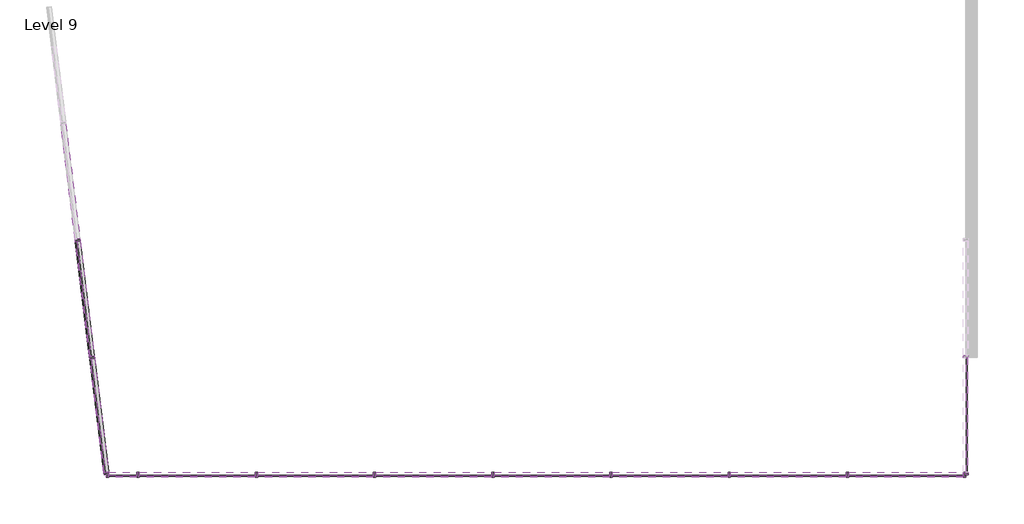
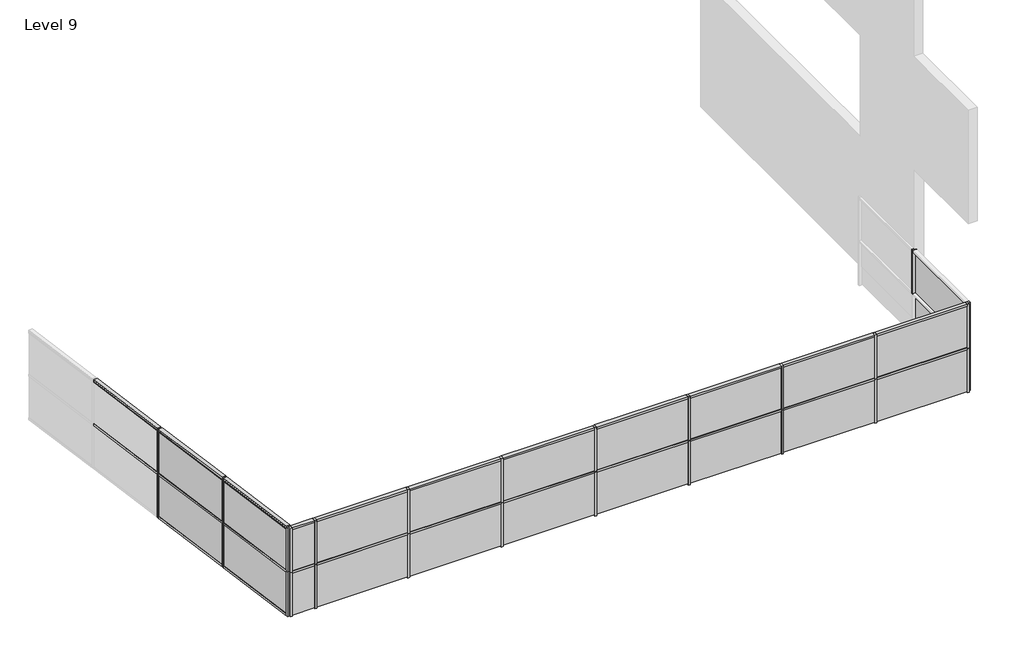
# One storey, part 1 of 2: 63 members, 26 plates.
"""IFC4 building model written with IfcOpenShell, lengths in millimetres."""

from ifc_helpers import new_model, si_unit, origin, place, context, project, spatial, transform, mapped, element, save
from components import member_71c27fd2, member_daa7a266, member_82905deb, member_19d0a4ec, member_8cef0660, member_db480205, member_4491d118, member_0c11e56c, member_695b83e4, system_panel_glazed_37f15d2e, system_panel_glazed_3620f98e, system_panel_glazed_e46d4b42, system_panel_glazed_2a6c68b7, system_panel_glazed_07b088f8, system_panel_glazed_9d0e0944

model = new_model("IFC4")

# Units and contexts
model_context = context("Model", 3, world=origin())
ifc_project = project(units=[si_unit("LENGTHUNIT", "METRE", prefix="MILLI")], contexts=[model_context])

# Site, building, storey
site = spatial("IfcSite", under=ifc_project)
building = spatial("IfcBuilding", under=site)
storey = spatial("IfcBuildingStorey", under=building, Name="Level 9", Elevation=24384.0)

# Members
placement = place(None, origin())
member_shape = member_71c27fd2(model_context)
element("IfcMember", 1, ObjectType="Rectangular Mullion : 2.5\" x 5\" rectangular", at=placement, inside=storey, context=model_context, shape_type="MappedRepresentation", body=[
    mapped(member_shape, transform((-8620.3262186, -3985.3690403, 24384.0), x_axis=(0.0, 0.0, -1.0), y_axis=(-0.9925461516413222, -0.12186934340514607, 0.0), z_axis=(-0.12186934340514607, 0.9925461516413222, 0.0))),
])
member_2_shape = member_daa7a266(model_context)
element("IfcMember", 2, ObjectType="Rectangular Mullion : 2.5\" x 5\" rectangular", at=placement, inside=storey, context=model_context, shape_type="MappedRepresentation", body=[
    mapped(member_2_shape, transform((13839.0156363, -6979.1363705, 27432.0), x_axis=(0.0, 0.0, 1.0), y_axis=(0.0, -1.0, 0.0), z_axis=(1.0, 0.0, 0.0))),
])
element("IfcMember", 3, ObjectType="Rectangular Mullion : 2.5\" x 5\" rectangular", at=placement, inside=storey, context=model_context, shape_type="MappedRepresentation", body=[
    mapped(member_2_shape, transform((-8260.4765148, -6916.1096898, 27432.0), x_axis=(0.0, 0.0, 1.0), y_axis=(-0.9925461516413222, -0.12186934340514587, 0.0), z_axis=(0.12186934340514587, -0.9925461516413222, 0.0))),
])
member_3_shape = member_82905deb(model_context)
element("IfcMember", 4, ObjectType="Rectangular Mullion : 2.5\" x 5\" rectangular", at=placement, inside=storey, context=model_context, shape_type="MappedRepresentation", body=[
    mapped(member_3_shape, transform((10854.515636, -6979.1363705, 27432.0), x_axis=(-1.0, 0.0, 0.0), y_axis=(0.0, -1.0, 0.0), z_axis=(0.0, 0.0, 1.0))),
])
element("IfcMember", 5, ObjectType="Rectangular Mullion : 2.5\" x 5\" rectangular", at=placement, inside=storey, context=model_context, shape_type="MappedRepresentation", body=[
    mapped(member_3_shape, transform((7806.515636, -6979.1363705, 27432.0), x_axis=(-1.0, 0.0, 0.0), y_axis=(0.0, -1.0, 0.0), z_axis=(0.0, 0.0, 1.0))),
])
element("IfcMember", 6, ObjectType="Rectangular Mullion : 2.5\" x 5\" rectangular", at=placement, inside=storey, context=model_context, shape_type="MappedRepresentation", body=[
    mapped(member_3_shape, transform((4758.515636, -6979.1363705, 27432.0), x_axis=(-1.0, 0.0, 0.0), y_axis=(0.0, -1.0, 0.0), z_axis=(0.0, 0.0, 1.0))),
])
element("IfcMember", 7, ObjectType="Rectangular Mullion : 2.5\" x 5\" rectangular", at=placement, inside=storey, context=model_context, shape_type="MappedRepresentation", body=[
    mapped(member_3_shape, transform((1710.515636, -6979.1363705, 27432.0), x_axis=(-1.0, 0.0, 0.0), y_axis=(0.0, -1.0, 0.0), z_axis=(0.0, 0.0, 1.0))),
])
element("IfcMember", 8, ObjectType="Rectangular Mullion : 2.5\" x 5\" rectangular", at=placement, inside=storey, context=model_context, shape_type="MappedRepresentation", body=[
    mapped(member_3_shape, transform((-1337.484364, -6979.1363705, 27432.0), x_axis=(-1.0, 0.0, 0.0), y_axis=(0.0, -1.0, 0.0), z_axis=(0.0, 0.0, 1.0))),
])
element("IfcMember", 9, ObjectType="Rectangular Mullion : 2.5\" x 5\" rectangular", at=placement, inside=storey, context=model_context, shape_type="MappedRepresentation", body=[
    mapped(member_3_shape, transform((-4385.484364, -6979.1363705, 27432.0), x_axis=(-1.0, 0.0, 0.0), y_axis=(0.0, -1.0, 0.0), z_axis=(0.0, 0.0, 1.0))),
])
element("IfcMember", 10, ObjectType="Rectangular Mullion : 2.5\" x 5\" rectangular", at=placement, inside=storey, context=model_context, shape_type="MappedRepresentation", body=[
    mapped(member_3_shape, transform((-7433.484364, -6979.1363705, 27432.0), x_axis=(-1.0, 0.0, 0.0), y_axis=(0.0, -1.0, 0.0), z_axis=(0.0, 0.0, 1.0))),
])
element("IfcMember", 11, ObjectType="Rectangular Mullion : 2.5\" x 5\" rectangular", at=placement, inside=storey, context=model_context, shape_type="MappedRepresentation", body=[
    mapped(member_3_shape, transform((-8624.1955702, -3953.8557, 27432.0), x_axis=(-0.1218693434051459, 0.9925461516413222, 0.0), y_axis=(-0.9925461516413222, -0.1218693434051459, 0.0), z_axis=(0.0, 0.0, 1.0))),
])
element("IfcMember", 12, ObjectType="Rectangular Mullion : 2.5\" x 5\" rectangular", at=placement, inside=storey, context=model_context, shape_type="MappedRepresentation", body=[
    mapped(member_3_shape, transform((-8995.6533289, -928.5750297, 27432.0), x_axis=(-0.1218693434051459, 0.9925461516413222, 0.0), y_axis=(-0.9925461516413222, -0.1218693434051459, 0.0), z_axis=(0.0, 0.0, 1.0))),
])
element("IfcMember", 13, ObjectType="Rectangular Mullion : 2.5\" x 5\" rectangular", at=placement, inside=storey, context=model_context, shape_type="MappedRepresentation", body=[
    mapped(member_3_shape, transform((13902.5156363, -3931.1363708, 27432.0), x_axis=(0.0, -1.0, 0.0), y_axis=(1.0, 0.0, 0.0), z_axis=(0.0, 0.0, 1.0))),
])
member_4_shape = member_19d0a4ec(model_context)
element("IfcMember", 14, ObjectType="Rectangular Mullion : 2.5\" x 5\" rectangular", at=placement, inside=storey, context=model_context, shape_type="MappedRepresentation", body=[
    mapped(member_4_shape, transform((13839.0156363, -6979.1363705, 25908.0), x_axis=(0.0, 0.0, 1.0), y_axis=(0.0, -1.0, 0.0), z_axis=(1.0, 0.0, 0.0))),
])
element("IfcMember", 15, ObjectType="Rectangular Mullion : 2.5\" x 5\" rectangular", at=placement, inside=storey, context=model_context, shape_type="MappedRepresentation", body=[
    mapped(member_4_shape, transform((-8260.4765148, -6916.1096898, 25908.0), x_axis=(0.0, 0.0, 1.0), y_axis=(-0.9925461516413222, -0.12186934340514595, 0.0), z_axis=(0.12186934340514595, -0.9925461516413222, 0.0))),
])
element("IfcMember", 16, ObjectType="Rectangular Mullion : 2.5\" x 5\" rectangular", at=placement, inside=storey, context=model_context, shape_type="MappedRepresentation", body=[
    mapped(member_4_shape, transform((-8260.4765148, -6916.1096898, 27432.0), x_axis=(0.0, 0.0, 1.0), y_axis=(-0.9925461516413223, -0.12186934340514578, 0.0), z_axis=(0.12186934340514578, -0.9925461516413223, 0.0))),
])
element("IfcMember", 17, ObjectType="Rectangular Mullion : 2.5\" x 5\" rectangular", at=placement, inside=storey, context=model_context, shape_type="MappedRepresentation", body=[
    mapped(member_4_shape, transform((-8260.4765148, -6916.1096898, 25908.0), x_axis=(0.0, 0.0, 1.0), y_axis=(-0.9925461516413222, -0.12186934340514567, 0.0), z_axis=(0.12186934340514567, -0.9925461516413222, 0.0))),
])
member_5_shape = member_8cef0660(model_context)
element("IfcMember", 18, ObjectType="Rectangular Mullion : 2.5\" x 5\" rectangular", at=placement, inside=storey, context=model_context, shape_type="MappedRepresentation", body=[
    mapped(member_5_shape, transform((10822.765636, -6979.1363705, 25908.0), x_axis=(0.0, 0.0, 1.0), y_axis=(0.0, -1.0, 0.0), z_axis=(1.0, 0.0, 0.0))),
])
element("IfcMember", 19, ObjectType="Rectangular Mullion : 2.5\" x 5\" rectangular", at=placement, inside=storey, context=model_context, shape_type="MappedRepresentation", body=[
    mapped(member_5_shape, transform((7774.765636, -6979.1363705, 25908.0), x_axis=(0.0, 0.0, 1.0), y_axis=(0.0, -1.0, 0.0), z_axis=(1.0, 0.0, 0.0))),
])
element("IfcMember", 20, ObjectType="Rectangular Mullion : 2.5\" x 5\" rectangular", at=placement, inside=storey, context=model_context, shape_type="MappedRepresentation", body=[
    mapped(member_5_shape, transform((4726.765636, -6979.1363705, 25908.0), x_axis=(0.0, 0.0, 1.0), y_axis=(0.0, -1.0, 0.0), z_axis=(1.0, 0.0, 0.0))),
])
element("IfcMember", 21, ObjectType="Rectangular Mullion : 2.5\" x 5\" rectangular", at=placement, inside=storey, context=model_context, shape_type="MappedRepresentation", body=[
    mapped(member_5_shape, transform((1678.765636, -6979.1363705, 25908.0), x_axis=(0.0, 0.0, 1.0), y_axis=(0.0, -1.0, 0.0), z_axis=(1.0, 0.0, 0.0))),
])
element("IfcMember", 22, ObjectType="Rectangular Mullion : 2.5\" x 5\" rectangular", at=placement, inside=storey, context=model_context, shape_type="MappedRepresentation", body=[
    mapped(member_5_shape, transform((-1369.234364, -6979.1363705, 25908.0), x_axis=(0.0, 0.0, 1.0), y_axis=(0.0, -1.0, 0.0), z_axis=(1.0, 0.0, 0.0))),
])
element("IfcMember", 23, ObjectType="Rectangular Mullion : 2.5\" x 5\" rectangular", at=placement, inside=storey, context=model_context, shape_type="MappedRepresentation", body=[
    mapped(member_5_shape, transform((-4417.234364, -6979.1363705, 25908.0), x_axis=(0.0, 0.0, 1.0), y_axis=(0.0, -1.0, 0.0), z_axis=(1.0, 0.0, 0.0))),
])
element("IfcMember", 24, ObjectType="Rectangular Mullion : 2.5\" x 5\" rectangular", at=placement, inside=storey, context=model_context, shape_type="MappedRepresentation", body=[
    mapped(member_5_shape, transform((-8628.0649219, -3922.3423596, 25908.0), x_axis=(0.0, 0.0, 1.0), y_axis=(-0.9925461516413222, -0.12186934340514592, 0.0), z_axis=(0.12186934340514592, -0.9925461516413222, 0.0))),
])
element("IfcMember", 25, ObjectType="Rectangular Mullion : 2.5\" x 5\" rectangular", at=placement, inside=storey, context=model_context, shape_type="MappedRepresentation", body=[
    mapped(member_5_shape, transform((-8999.5226806, -897.0616894, 25908.0), x_axis=(0.0, 0.0, 1.0), y_axis=(-0.9925461516413222, -0.12186934340514566, 0.0), z_axis=(0.12186934340514566, -0.9925461516413222, 0.0))),
])
element("IfcMember", 26, ObjectType="Rectangular Mullion : 2.5\" x 5\" rectangular", at=placement, inside=storey, context=model_context, shape_type="MappedRepresentation", body=[
    mapped(member_5_shape, transform((-8628.0649219, -3922.3423596, 27432.0), x_axis=(0.0, 0.0, 1.0), y_axis=(-0.9925461516413222, -0.12186934340514592, 0.0), z_axis=(0.12186934340514592, -0.9925461516413222, 0.0))),
])
element("IfcMember", 27, ObjectType="Rectangular Mullion : 2.5\" x 5\" rectangular", at=placement, inside=storey, context=model_context, shape_type="MappedRepresentation", body=[
    mapped(member_5_shape, transform((-8999.5226806, -897.0616894, 27432.0), x_axis=(0.0, 0.0, 1.0), y_axis=(-0.9925461516413222, -0.12186934340514602, 0.0), z_axis=(0.12186934340514602, -0.9925461516413222, 0.0))),
])
element("IfcMember", 28, ObjectType="Rectangular Mullion : 2.5\" x 5\" rectangular", at=placement, inside=storey, context=model_context, shape_type="MappedRepresentation", body=[
    mapped(member_5_shape, transform((-8628.0649219, -3922.3423596, 25908.0), x_axis=(0.0, 0.0, 1.0), y_axis=(-0.9925461516413222, -0.12186934340514603, 0.0), z_axis=(0.12186934340514603, -0.9925461516413222, 0.0))),
])
element("IfcMember", 29, ObjectType="Rectangular Mullion : 2.5\" x 5\" rectangular", at=placement, inside=storey, context=model_context, shape_type="MappedRepresentation", body=[
    mapped(member_5_shape, transform((-8999.5226806, -897.0616894, 25908.0), x_axis=(0.0, 0.0, 1.0), y_axis=(-0.9925461516413222, -0.12186934340514596, 0.0), z_axis=(0.12186934340514596, -0.9925461516413222, 0.0))),
])
member_6_shape = member_db480205(model_context)
element("IfcMember", 30, ObjectType="Rectangular Mullion : 2.5\" x 5\" rectangular", at=placement, inside=storey, context=model_context, shape_type="MappedRepresentation", body=[
    mapped(member_6_shape, transform((-8991.7839773, -960.0883701, 24384.0), x_axis=(0.0, 0.0, -1.0), y_axis=(-0.9925461516413222, -0.12186934340514592, 0.0), z_axis=(-0.12186934340514592, 0.9925461516413222, 0.0))),
])
element("IfcMember", 31, ObjectType="Rectangular Mullion : 2.5\" x 5\" rectangular", at=placement, inside=storey, context=model_context, shape_type="MappedRepresentation", body=[
    mapped(member_6_shape, transform((10822.765636, -6979.1363705, 27432.0), x_axis=(0.0, 0.0, 1.0), y_axis=(0.0, -1.0, 0.0), z_axis=(1.0, 0.0, 0.0))),
])
element("IfcMember", 32, ObjectType="Rectangular Mullion : 2.5\" x 5\" rectangular", at=placement, inside=storey, context=model_context, shape_type="MappedRepresentation", body=[
    mapped(member_6_shape, transform((7774.765636, -6979.1363705, 27432.0), x_axis=(0.0, 0.0, 1.0), y_axis=(0.0, -1.0, 0.0), z_axis=(1.0, 0.0, 0.0))),
])
element("IfcMember", 33, ObjectType="Rectangular Mullion : 2.5\" x 5\" rectangular", at=placement, inside=storey, context=model_context, shape_type="MappedRepresentation", body=[
    mapped(member_6_shape, transform((4726.765636, -6979.1363705, 27432.0), x_axis=(0.0, 0.0, 1.0), y_axis=(0.0, -1.0, 0.0), z_axis=(1.0, 0.0, 0.0))),
])
element("IfcMember", 34, ObjectType="Rectangular Mullion : 2.5\" x 5\" rectangular", at=placement, inside=storey, context=model_context, shape_type="MappedRepresentation", body=[
    mapped(member_6_shape, transform((1678.765636, -6979.1363705, 27432.0), x_axis=(0.0, 0.0, 1.0), y_axis=(0.0, -1.0, 0.0), z_axis=(1.0, 0.0, 0.0))),
])
element("IfcMember", 35, ObjectType="Rectangular Mullion : 2.5\" x 5\" rectangular", at=placement, inside=storey, context=model_context, shape_type="MappedRepresentation", body=[
    mapped(member_6_shape, transform((-1369.234364, -6979.1363705, 27432.0), x_axis=(0.0, 0.0, 1.0), y_axis=(0.0, -1.0, 0.0), z_axis=(1.0, 0.0, 0.0))),
])
element("IfcMember", 36, ObjectType="Rectangular Mullion : 2.5\" x 5\" rectangular", at=placement, inside=storey, context=model_context, shape_type="MappedRepresentation", body=[
    mapped(member_6_shape, transform((-4417.234364, -6979.1363705, 27432.0), x_axis=(0.0, 0.0, 1.0), y_axis=(0.0, -1.0, 0.0), z_axis=(1.0, 0.0, 0.0))),
])
element("IfcMember", 37, ObjectType="Rectangular Mullion : 2.5\" x 5\" rectangular", at=placement, inside=storey, context=model_context, shape_type="MappedRepresentation", body=[
    mapped(member_6_shape, transform((-8628.0649219, -3922.3423596, 27432.0), x_axis=(0.0, 0.0, 1.0), y_axis=(-0.9925461516413222, -0.12186934340514599, 0.0), z_axis=(0.12186934340514599, -0.9925461516413222, 0.0))),
])
element("IfcMember", 38, ObjectType="Rectangular Mullion : 2.5\" x 5\" rectangular", at=placement, inside=storey, context=model_context, shape_type="MappedRepresentation", body=[
    mapped(member_6_shape, transform((-8999.5226806, -897.0616894, 27432.0), x_axis=(0.0, 0.0, 1.0), y_axis=(-0.9925461516413222, -0.12186934340514596, 0.0), z_axis=(0.12186934340514596, -0.9925461516413222, 0.0))),
])
element("IfcMember", 39, ObjectType="Rectangular Mullion : 2.5\" x 5\" rectangular", at=placement, inside=storey, context=model_context, shape_type="MappedRepresentation", body=[
    mapped(member_3_shape, transform((-8624.1955702, -3953.8557, 25908.0), x_axis=(-0.1218693434051459, 0.9925461516413222, 0.0), y_axis=(-0.9925461516413222, -0.1218693434051459, 0.0), z_axis=(0.0, 0.0, 1.0))),
])
element("IfcMember", 40, ObjectType="Rectangular Mullion : 2.5\" x 5\" rectangular", at=placement, inside=storey, context=model_context, shape_type="MappedRepresentation", body=[
    mapped(member_3_shape, transform((-8995.6533289, -928.5750297, 25908.0), x_axis=(-0.1218693434051459, 0.9925461516413222, 0.0), y_axis=(-0.9925461516413222, -0.1218693434051459, 0.0), z_axis=(0.0, 0.0, 1.0))),
])
element("IfcMember", 41, ObjectType="Rectangular Mullion : 2.5\" x 5\" rectangular", at=placement, inside=storey, context=model_context, shape_type="MappedRepresentation", body=[
    mapped(member_3_shape, transform((10854.515636, -6979.1363705, 25908.0), x_axis=(-1.0, 0.0, 0.0), y_axis=(0.0, -1.0, 0.0), z_axis=(0.0, 0.0, 1.0))),
])
element("IfcMember", 42, ObjectType="Rectangular Mullion : 2.5\" x 5\" rectangular", at=placement, inside=storey, context=model_context, shape_type="MappedRepresentation", body=[
    mapped(member_3_shape, transform((7806.515636, -6979.1363705, 25908.0), x_axis=(-1.0, 0.0, 0.0), y_axis=(0.0, -1.0, 0.0), z_axis=(0.0, 0.0, 1.0))),
])
element("IfcMember", 43, ObjectType="Rectangular Mullion : 2.5\" x 5\" rectangular", at=placement, inside=storey, context=model_context, shape_type="MappedRepresentation", body=[
    mapped(member_3_shape, transform((4758.515636, -6979.1363705, 25908.0), x_axis=(-1.0, 0.0, 0.0), y_axis=(0.0, -1.0, 0.0), z_axis=(0.0, 0.0, 1.0))),
])
element("IfcMember", 44, ObjectType="Rectangular Mullion : 2.5\" x 5\" rectangular", at=placement, inside=storey, context=model_context, shape_type="MappedRepresentation", body=[
    mapped(member_3_shape, transform((1710.515636, -6979.1363705, 25908.0), x_axis=(-1.0, 0.0, 0.0), y_axis=(0.0, -1.0, 0.0), z_axis=(0.0, 0.0, 1.0))),
])
element("IfcMember", 45, ObjectType="Rectangular Mullion : 2.5\" x 5\" rectangular", at=placement, inside=storey, context=model_context, shape_type="MappedRepresentation", body=[
    mapped(member_3_shape, transform((-1337.484364, -6979.1363705, 25908.0), x_axis=(-1.0, 0.0, 0.0), y_axis=(0.0, -1.0, 0.0), z_axis=(0.0, 0.0, 1.0))),
])
element("IfcMember", 46, ObjectType="Rectangular Mullion : 2.5\" x 5\" rectangular", at=placement, inside=storey, context=model_context, shape_type="MappedRepresentation", body=[
    mapped(member_3_shape, transform((-4385.484364, -6979.1363705, 25908.0), x_axis=(-1.0, 0.0, 0.0), y_axis=(0.0, -1.0, 0.0), z_axis=(0.0, 0.0, 1.0))),
])
element("IfcMember", 47, ObjectType="Rectangular Mullion : 2.5\" x 5\" rectangular", at=placement, inside=storey, context=model_context, shape_type="MappedRepresentation", body=[
    mapped(member_3_shape, transform((-7433.484364, -6979.1363705, 25908.0), x_axis=(-1.0, 0.0, 0.0), y_axis=(0.0, -1.0, 0.0), z_axis=(0.0, 0.0, 1.0))),
])
element("IfcMember", 48, ObjectType="Rectangular Mullion : 2.5\" x 5\" rectangular", at=placement, inside=storey, context=model_context, shape_type="MappedRepresentation", body=[
    mapped(member_3_shape, transform((-8624.1955702, -3953.8557, 27432.0), x_axis=(-0.1218693434051459, 0.9925461516413222, 0.0), y_axis=(-0.9925461516413222, -0.1218693434051459, 0.0), z_axis=(0.0, 0.0, 1.0))),
])
element("IfcMember", 49, ObjectType="Rectangular Mullion : 2.5\" x 5\" rectangular", at=placement, inside=storey, context=model_context, shape_type="MappedRepresentation", body=[
    mapped(member_3_shape, transform((-8995.6533289, -928.5750297, 27432.0), x_axis=(-0.1218693434051459, 0.9925461516413222, 0.0), y_axis=(-0.9925461516413222, -0.1218693434051459, 0.0), z_axis=(0.0, 0.0, 1.0))),
])
element("IfcMember", 50, ObjectType="Rectangular Mullion : 2.5\" x 5\" rectangular", at=placement, inside=storey, context=model_context, shape_type="MappedRepresentation", body=[
    mapped(member_3_shape, transform((-8624.1955702, -3953.8557, 25908.0), x_axis=(-0.1218693434051459, 0.9925461516413222, 0.0), y_axis=(-0.9925461516413222, -0.1218693434051459, 0.0), z_axis=(0.0, 0.0, 1.0))),
])
element("IfcMember", 51, ObjectType="Rectangular Mullion : 2.5\" x 5\" rectangular", at=placement, inside=storey, context=model_context, shape_type="MappedRepresentation", body=[
    mapped(member_3_shape, transform((-8995.6533289, -928.5750297, 25908.0), x_axis=(-0.1218693434051459, 0.9925461516413222, 0.0), y_axis=(-0.9925461516413222, -0.1218693434051459, 0.0), z_axis=(0.0, 0.0, 1.0))),
])
member_7_shape = member_4491d118(model_context)
element("IfcMember", 52, ObjectType="Rectangular Mullion : 2.5\" x 5\" rectangular", at=placement, inside=storey, context=model_context, shape_type="MappedRepresentation", body=[
    mapped(member_7_shape, transform((-8252.7378115, -6979.1363705, 27432.0), x_axis=(-1.0, 0.0, 0.0), y_axis=(0.0, -1.0, 0.0), z_axis=(0.0, 0.0, 1.0))),
])
element("IfcMember", 53, ObjectType="Rectangular Mullion : 2.5\" x 5\" rectangular", at=placement, inside=storey, context=model_context, shape_type="MappedRepresentation", body=[
    mapped(member_7_shape, transform((13902.5156363, -6979.1363705, 27432.0), x_axis=(0.0, -1.0, 0.0), y_axis=(1.0, 0.0, 0.0), z_axis=(0.0, 0.0, 1.0))),
])
element("IfcMember", 54, ObjectType="Rectangular Mullion : 2.5\" x 5\" rectangular", at=placement, inside=storey, context=model_context, shape_type="MappedRepresentation", body=[
    mapped(member_7_shape, transform((-8252.7378115, -6979.1363705, 24384.0), x_axis=(0.1218693434051459, -0.9925461516413222, 0.0), y_axis=(-0.9925461516413222, -0.1218693434051459, 0.0), z_axis=(0.0, 0.0, -1.0))),
])
element("IfcMember", 55, ObjectType="Rectangular Mullion : 2.5\" x 5\" rectangular", at=placement, inside=storey, context=model_context, shape_type="MappedRepresentation", body=[
    mapped(member_7_shape, transform((13902.5156363, -6979.1363705, 24384.0), x_axis=(1.0, 0.0, 0.0), y_axis=(0.0, -1.0, 0.0), z_axis=(0.0, 0.0, -1.0))),
])
element("IfcMember", 56, ObjectType="Rectangular Mullion : 2.5\" x 5\" rectangular", at=placement, inside=storey, context=model_context, shape_type="MappedRepresentation", body=[
    mapped(member_7_shape, transform((-8252.7378115, -6979.1363705, 25908.0), x_axis=(0.1218693434051459, -0.9925461516413222, 0.0), y_axis=(-0.9925461516413222, -0.1218693434051459, 0.0), z_axis=(0.0, 0.0, -1.0))),
])
element("IfcMember", 57, ObjectType="Rectangular Mullion : 2.5\" x 5\" rectangular", at=placement, inside=storey, context=model_context, shape_type="MappedRepresentation", body=[
    mapped(member_7_shape, transform((-8252.7378115, -6979.1363705, 24384.0), x_axis=(0.1218693434051459, -0.9925461516413222, 0.0), y_axis=(-0.9925461516413222, -0.1218693434051459, 0.0), z_axis=(0.0, 0.0, -1.0))),
])
element("IfcMember", 58, ObjectType="Rectangular Mullion : 2.5\" x 5\" rectangular", at=placement, inside=storey, context=model_context, shape_type="MappedRepresentation", body=[
    mapped(member_7_shape, transform((13902.5156363, -6979.1363705, 25908.0), x_axis=(1.0, 0.0, 0.0), y_axis=(0.0, -1.0, 0.0), z_axis=(0.0, 0.0, -1.0))),
])
element("IfcMember", 59, ObjectType="Rectangular Mullion : 2.5\" x 5\" rectangular", at=placement, inside=storey, context=model_context, shape_type="MappedRepresentation", body=[
    mapped(member_7_shape, transform((-8252.7378115, -6979.1363705, 25908.0), x_axis=(0.1218693434051459, -0.9925461516413222, 0.0), y_axis=(-0.9925461516413222, -0.1218693434051459, 0.0), z_axis=(0.0, 0.0, -1.0))),
])
element("IfcMember", 60, ObjectType="Rectangular Mullion : 2.5\" x 5\" rectangular", at=placement, inside=storey, context=model_context, shape_type="MappedRepresentation", body=[
    mapped(member_7_shape, transform((-8252.7378115, -6979.1363705, 25908.0), x_axis=(-1.0, 0.0, 0.0), y_axis=(0.0, -1.0, 0.0), z_axis=(0.0, 0.0, 1.0))),
])
element("IfcMember", 61, ObjectType="Rectangular Mullion : 2.5\" x 5\" rectangular", at=placement, inside=storey, context=model_context, shape_type="MappedRepresentation", body=[
    mapped(member_7_shape, transform((13902.5156363, -6979.1363705, 25908.0), x_axis=(0.0, -1.0, 0.0), y_axis=(1.0, 0.0, 0.0), z_axis=(0.0, 0.0, 1.0))),
])
member_8_shape = member_0c11e56c(model_context)
element("IfcMember", 62, ObjectType="Rectangular Mullion : 2.5\" x 5\" rectangular", at=placement, inside=storey, context=model_context, shape_type="MappedRepresentation", body=[
    mapped(member_8_shape, transform((-7465.234364, -6979.1363705, 25908.0), x_axis=(0.0, 0.0, 1.0), y_axis=(0.0, -1.0, 0.0), z_axis=(1.0, 0.0, 0.0))),
])
member_9_shape = member_695b83e4(model_context)
element("IfcMember", 63, ObjectType="Rectangular Mullion : 2.5\" x 5\" rectangular", at=placement, inside=storey, context=model_context, shape_type="MappedRepresentation", body=[
    mapped(member_9_shape, transform((-7465.234364, -6979.1363705, 27432.0), x_axis=(0.0, 0.0, 1.0), y_axis=(0.0, -1.0, 0.0), z_axis=(1.0, 0.0, 0.0))),
])

# Plates
system_panel_glazed_shape = system_panel_glazed_37f15d2e(model_context)
element("IfcPlate", 64, ObjectType="System Panel : Glazed", at=placement, inside=storey, context=model_context, shape_type="MappedRepresentation", body=[
    mapped(system_panel_glazed_shape, transform((-8440.4013667, -5450.739365, 24447.5), x_axis=(-0.1218693434051459, 0.9925461516413222, 0.0), y_axis=(-0.9925461516413222, -0.1218693434051459, 0.0), z_axis=(0.0, 0.0, 1.0))),
])
element("IfcPlate", 65, ObjectType="System Panel : Glazed", at=placement, inside=storey, context=model_context, shape_type="MappedRepresentation", body=[
    mapped(system_panel_glazed_shape, transform((-8440.4013667, -5450.739365, 25939.75), x_axis=(-0.1218693434051459, 0.9925461516413222, 0.0), y_axis=(-0.9925461516413222, -0.1218693434051459, 0.0), z_axis=(0.0, 0.0, 1.0))),
])
element("IfcPlate", 66, ObjectType="System Panel : Glazed", at=placement, inside=storey, context=model_context, shape_type="MappedRepresentation", body=[
    mapped(system_panel_glazed_shape, transform((12362.6406361, -6979.1363705, 25939.75), x_axis=(-1.0, 0.0, 0.0), y_axis=(0.0, -1.0, 0.0), z_axis=(0.0, 0.0, 1.0))),
])
element("IfcPlate", 67, ObjectType="System Panel : Glazed", at=placement, inside=storey, context=model_context, shape_type="MappedRepresentation", body=[
    mapped(system_panel_glazed_shape, transform((13902.5156363, -5439.2613706, 25939.75), x_axis=(0.0, -1.0, 0.0), y_axis=(1.0, 0.0, 0.0), z_axis=(0.0, 0.0, 1.0))),
])
system_panel_glazed_2_shape = system_panel_glazed_3620f98e(model_context)
element("IfcPlate", 68, ObjectType="System Panel : Glazed", at=placement, inside=storey, context=model_context, shape_type="MappedRepresentation", body=[
    mapped(system_panel_glazed_2_shape, transform((-8809.9244496, -2441.2153649, 25939.75), x_axis=(-0.1218693434051459, 0.9925461516413222, 0.0), y_axis=(-0.9925461516413222, -0.1218693434051459, 0.0), z_axis=(0.0, 0.0, 1.0))),
])
element("IfcPlate", 69, ObjectType="System Panel : Glazed", at=placement, inside=storey, context=model_context, shape_type="MappedRepresentation", body=[
    mapped(system_panel_glazed_2_shape, transform((9330.515636, -6979.1363705, 25939.75), x_axis=(-1.0, 0.0, 0.0), y_axis=(0.0, -1.0, 0.0), z_axis=(0.0, 0.0, 1.0))),
])
element("IfcPlate", 70, ObjectType="System Panel : Glazed", at=placement, inside=storey, context=model_context, shape_type="MappedRepresentation", body=[
    mapped(system_panel_glazed_2_shape, transform((6282.515636, -6979.1363705, 25939.75), x_axis=(-1.0, 0.0, 0.0), y_axis=(0.0, -1.0, 0.0), z_axis=(0.0, 0.0, 1.0))),
])
element("IfcPlate", 71, ObjectType="System Panel : Glazed", at=placement, inside=storey, context=model_context, shape_type="MappedRepresentation", body=[
    mapped(system_panel_glazed_2_shape, transform((3234.515636, -6979.1363705, 25939.75), x_axis=(-1.0, 0.0, 0.0), y_axis=(0.0, -1.0, 0.0), z_axis=(0.0, 0.0, 1.0))),
])
element("IfcPlate", 72, ObjectType="System Panel : Glazed", at=placement, inside=storey, context=model_context, shape_type="MappedRepresentation", body=[
    mapped(system_panel_glazed_2_shape, transform((186.515636, -6979.1363705, 25939.75), x_axis=(-1.0, 0.0, 0.0), y_axis=(0.0, -1.0, 0.0), z_axis=(0.0, 0.0, 1.0))),
])
element("IfcPlate", 73, ObjectType="System Panel : Glazed", at=placement, inside=storey, context=model_context, shape_type="MappedRepresentation", body=[
    mapped(system_panel_glazed_2_shape, transform((-2861.484364, -6979.1363705, 25939.75), x_axis=(-1.0, 0.0, 0.0), y_axis=(0.0, -1.0, 0.0), z_axis=(0.0, 0.0, 1.0))),
])
element("IfcPlate", 74, ObjectType="System Panel : Glazed", at=placement, inside=storey, context=model_context, shape_type="MappedRepresentation", body=[
    mapped(system_panel_glazed_2_shape, transform((-5909.484364, -6979.1363705, 25939.75), x_axis=(-1.0, 0.0, 0.0), y_axis=(0.0, -1.0, 0.0), z_axis=(0.0, 0.0, 1.0))),
])
element("IfcPlate", 75, ObjectType="System Panel : Glazed", at=placement, inside=storey, context=model_context, shape_type="MappedRepresentation", body=[
    mapped(system_panel_glazed_2_shape, transform((-8809.9244496, -2441.2153649, 24447.5), x_axis=(-0.1218693434051459, 0.9925461516413222, 0.0), y_axis=(-0.9925461516413222, -0.1218693434051459, 0.0), z_axis=(0.0, 0.0, 1.0))),
])
system_panel_glazed_3_shape = system_panel_glazed_e46d4b42(model_context)
element("IfcPlate", 76, ObjectType="System Panel : Glazed", at=placement, inside=storey, context=model_context, shape_type="MappedRepresentation", body=[
    mapped(system_panel_glazed_3_shape, transform((-8440.4013667, -5450.739365, 24415.75), x_axis=(-0.1218693434051459, 0.9925461516413222, 0.0), y_axis=(-0.9925461516413222, -0.1218693434051459, 0.0), z_axis=(0.0, 0.0, 1.0))),
])
element("IfcPlate", 77, ObjectType="System Panel : Glazed", at=placement, inside=storey, context=model_context, shape_type="MappedRepresentation", body=[
    mapped(system_panel_glazed_3_shape, transform((12362.6406361, -6979.1363705, 24415.75), x_axis=(-1.0, 0.0, 0.0), y_axis=(0.0, -1.0, 0.0), z_axis=(0.0, 0.0, 1.0))),
])
element("IfcPlate", 78, ObjectType="System Panel : Glazed", at=placement, inside=storey, context=model_context, shape_type="MappedRepresentation", body=[
    mapped(system_panel_glazed_3_shape, transform((13902.5156363, -5439.2613706, 24415.75), x_axis=(0.0, -1.0, 0.0), y_axis=(1.0, 0.0, 0.0), z_axis=(0.0, 0.0, 1.0))),
])
element("IfcPlate", 79, ObjectType="System Panel : Glazed", at=placement, inside=storey, context=model_context, shape_type="MappedRepresentation", body=[
    mapped(system_panel_glazed_3_shape, transform((-8440.4013667, -5450.739365, 25939.75), x_axis=(-0.1218693434051459, 0.9925461516413222, 0.0), y_axis=(-0.9925461516413222, -0.1218693434051459, 0.0), z_axis=(0.0, 0.0, 1.0))),
])
system_panel_glazed_4_shape = system_panel_glazed_2a6c68b7(model_context)
element("IfcPlate", 80, ObjectType="System Panel : Glazed", at=placement, inside=storey, context=model_context, shape_type="MappedRepresentation", body=[
    mapped(system_panel_glazed_4_shape, transform((-8809.9244496, -2441.2153649, 24415.75), x_axis=(-0.1218693434051459, 0.9925461516413222, 0.0), y_axis=(-0.9925461516413222, -0.1218693434051459, 0.0), z_axis=(0.0, 0.0, 1.0))),
])
element("IfcPlate", 81, ObjectType="System Panel : Glazed", at=placement, inside=storey, context=model_context, shape_type="MappedRepresentation", body=[
    mapped(system_panel_glazed_4_shape, transform((9330.515636, -6979.1363705, 24415.75), x_axis=(-1.0, 0.0, 0.0), y_axis=(0.0, -1.0, 0.0), z_axis=(0.0, 0.0, 1.0))),
])
element("IfcPlate", 82, ObjectType="System Panel : Glazed", at=placement, inside=storey, context=model_context, shape_type="MappedRepresentation", body=[
    mapped(system_panel_glazed_4_shape, transform((6282.515636, -6979.1363705, 24415.75), x_axis=(-1.0, 0.0, 0.0), y_axis=(0.0, -1.0, 0.0), z_axis=(0.0, 0.0, 1.0))),
])
element("IfcPlate", 83, ObjectType="System Panel : Glazed", at=placement, inside=storey, context=model_context, shape_type="MappedRepresentation", body=[
    mapped(system_panel_glazed_4_shape, transform((3234.515636, -6979.1363705, 24415.75), x_axis=(-1.0, 0.0, 0.0), y_axis=(0.0, -1.0, 0.0), z_axis=(0.0, 0.0, 1.0))),
])
element("IfcPlate", 84, ObjectType="System Panel : Glazed", at=placement, inside=storey, context=model_context, shape_type="MappedRepresentation", body=[
    mapped(system_panel_glazed_4_shape, transform((186.515636, -6979.1363705, 24415.75), x_axis=(-1.0, 0.0, 0.0), y_axis=(0.0, -1.0, 0.0), z_axis=(0.0, 0.0, 1.0))),
])
element("IfcPlate", 85, ObjectType="System Panel : Glazed", at=placement, inside=storey, context=model_context, shape_type="MappedRepresentation", body=[
    mapped(system_panel_glazed_4_shape, transform((-2861.484364, -6979.1363705, 24415.75), x_axis=(-1.0, 0.0, 0.0), y_axis=(0.0, -1.0, 0.0), z_axis=(0.0, 0.0, 1.0))),
])
element("IfcPlate", 86, ObjectType="System Panel : Glazed", at=placement, inside=storey, context=model_context, shape_type="MappedRepresentation", body=[
    mapped(system_panel_glazed_4_shape, transform((-5909.484364, -6979.1363705, 24415.75), x_axis=(-1.0, 0.0, 0.0), y_axis=(0.0, -1.0, 0.0), z_axis=(0.0, 0.0, 1.0))),
])
element("IfcPlate", 87, ObjectType="System Panel : Glazed", at=placement, inside=storey, context=model_context, shape_type="MappedRepresentation", body=[
    mapped(system_panel_glazed_4_shape, transform((-8809.9244496, -2441.2153649, 25939.75), x_axis=(-0.1218693434051459, 0.9925461516413222, 0.0), y_axis=(-0.9925461516413222, -0.1218693434051459, 0.0), z_axis=(0.0, 0.0, 1.0))),
])
system_panel_glazed_5_shape = system_panel_glazed_07b088f8(model_context)
element("IfcPlate", 88, ObjectType="System Panel : Glazed", at=placement, inside=storey, context=model_context, shape_type="MappedRepresentation", body=[
    mapped(system_panel_glazed_5_shape, transform((-7827.2360878, -6979.1363705, 25939.75), x_axis=(-1.0, 0.0, 0.0), y_axis=(0.0, -1.0, 0.0), z_axis=(0.0, 0.0, 1.0))),
])
system_panel_glazed_6_shape = system_panel_glazed_9d0e0944(model_context)
element("IfcPlate", 89, ObjectType="System Panel : Glazed", at=placement, inside=storey, context=model_context, shape_type="MappedRepresentation", body=[
    mapped(system_panel_glazed_6_shape, transform((-7827.2360878, -6979.1363705, 24415.75), x_axis=(-1.0, 0.0, 0.0), y_axis=(0.0, -1.0, 0.0), z_axis=(0.0, 0.0, 1.0))),
])

save(model, "model.ifc")

# Revit data of these elements
# Type "Rectangular Mullion : 2.5\" x 5\" rectangular"
#   built-in parameter 1007304 = 0.416667 (stored number, unit not read)
#   built-in parameter 1007301 = 0.104167 (stored number, unit not read)
#   built-in parameter 1007300 = 0.104167 (stored number, unit not read)
# Type "System Panel : Glazed"
#   Construction Type Id = "GSP4R"
#   Analytic Construction = "1/8 in Pilkington single glazing"
#   Visual Light Transmittance = 0.9
#   Solar Heat Gain Coefficient = 0.86
#   Heat Transfer Coefficient (U) = 1.18115 BTU/(h·ft²·°F)
#   Define Thermal Properties by = 1
# Elements 1, 2, 3, 4, 5, 6, 7, 8, 9, 10, 11, 12, 13, 14, 15, 16, 17, 18, 19, 20, 21, 22, 23, 24, 25, 26, 27, 28, 29, 30, 31, 32, 33, 34, 35, 36, 37, 38, 39, 40, 41, 42, 43, 44, 45, 46, 47, 48, 49, 50, 51, 52, 53, 54, 55, 56, 57, 58, 59, 60, 61, 62, 63 (IfcMember, "Rectangular Mullion : 2.5\" x 5\" rectangular")
#   Phase Created = New Construction
#   Materials on its faces: "Aluminum"
# Elements 64, 65, 66, 67, 68, 69, 70, 71, 72, 73, 74, 75, 76, 77, 78, 79, 80, 81, 82, 83, 84, 85, 86, 87, 88, 89 (IfcPlate, "System Panel : Glazed")
#   Phase Created = New Construction
#   Materials on its faces: "Glass"
# Materials
#   "Aluminum": class "Metal", colour RGB 247 247 247, transparency 0, Description = "Aluminum 6061", Cost = 0
#   "Glass": class "Glass", colour RGB 0 128 192, transparency 0.75, Description = "Soda Lime Glass", Cost = 0
